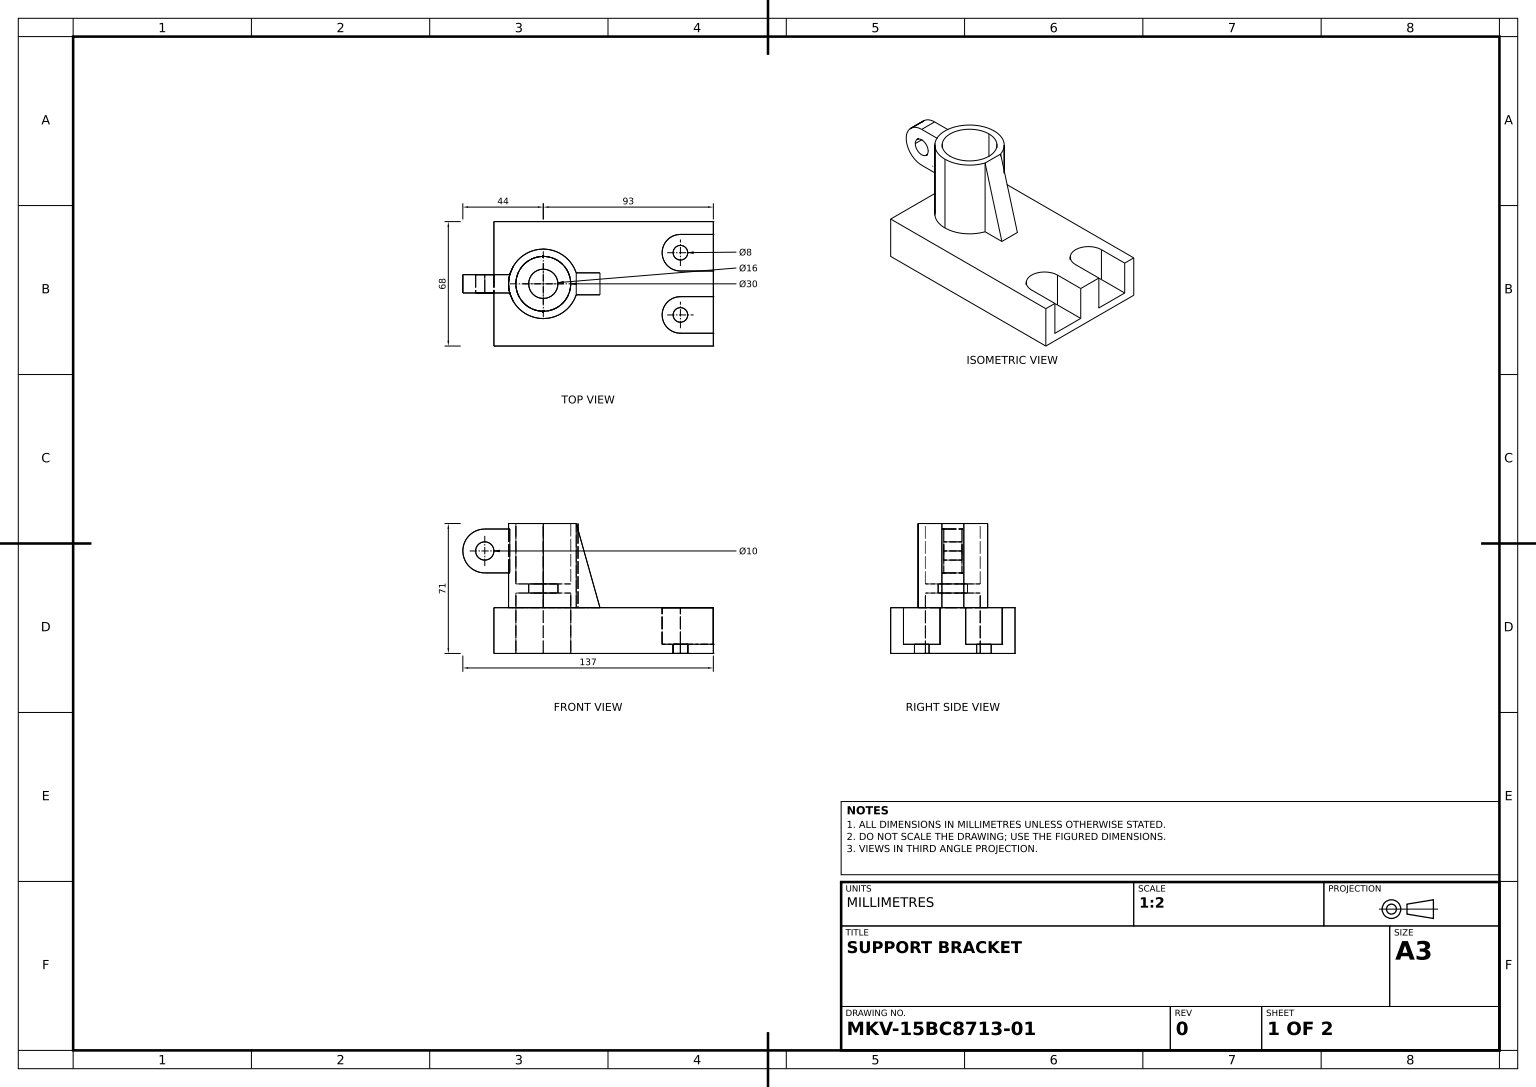
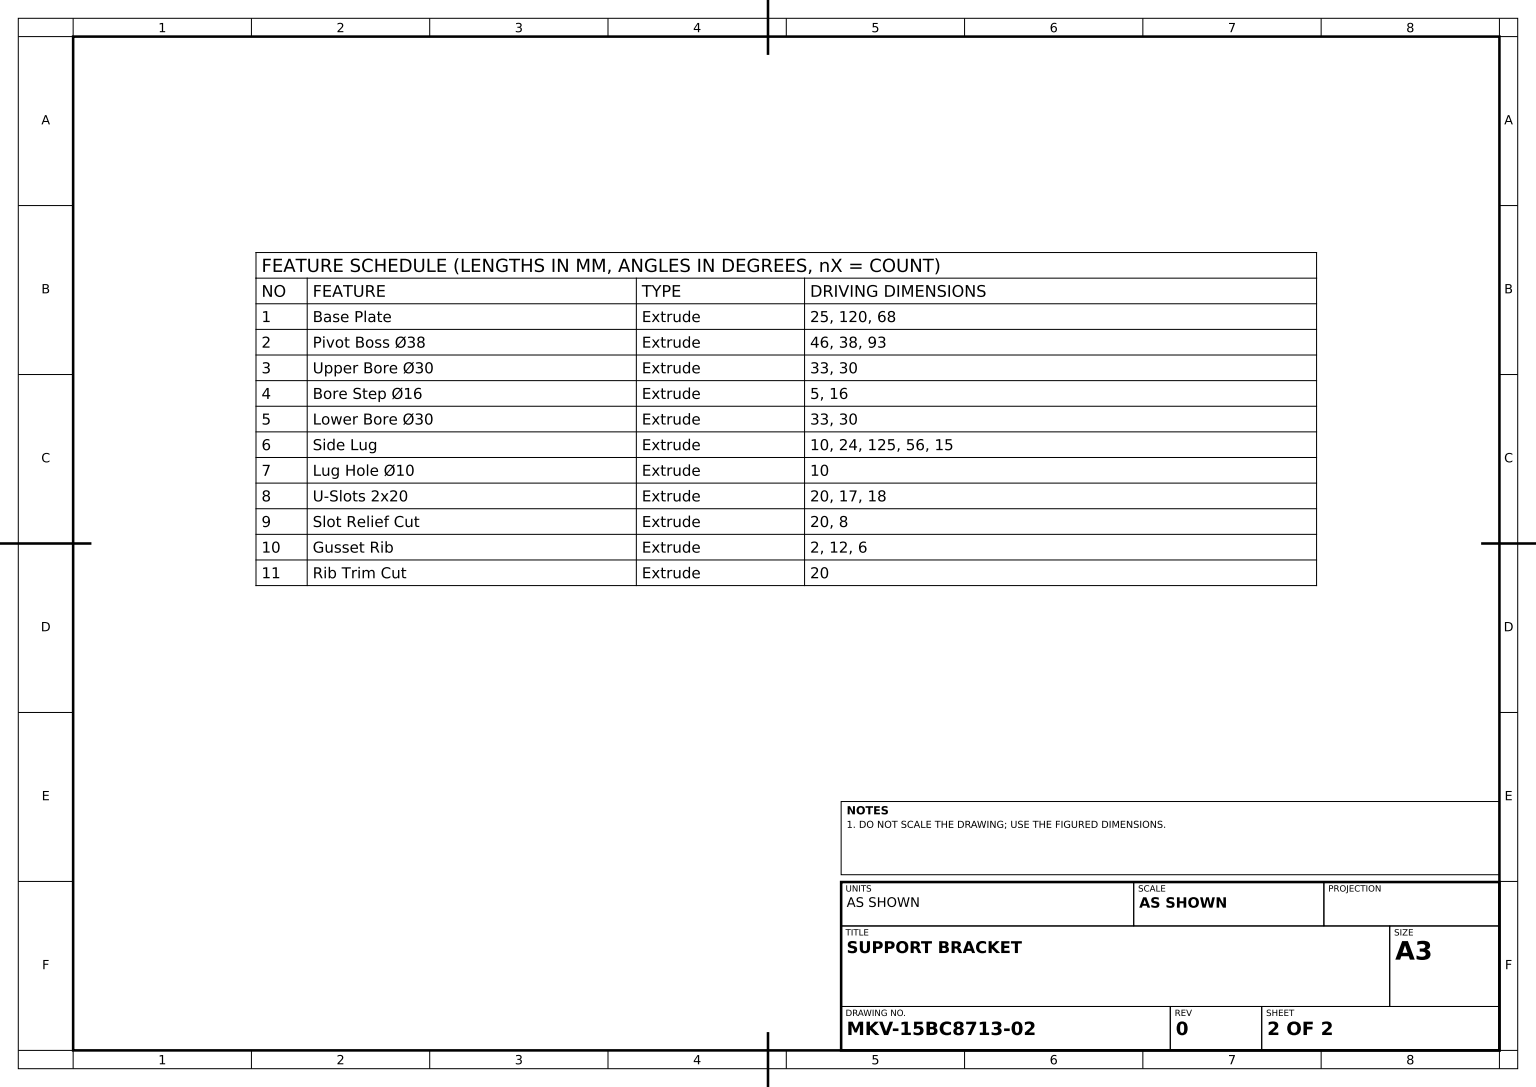
SolidWorks part; units mm, degrees
material "Plain Carbon Steel"
ref_plane "Front Plane" through (0, 0, 0) normal (0, 0, 1) x (1, 0, 0)
ref_plane "Top Plane" through (0, 0, 0) normal (0, 1, 0) x (1, 0, 0)
ref_plane "Right Plane" through (0, 0, 0) normal (1, 0, 0) x (0, 0, -1)
sketch "Base Plate Sketch" plane through (0, 0, 0) normal (0, 1, 0) x (1, 0, 0)
  line L1 (-60, -34) -> (60, -34)
  line L2 (-60, -34) -> (-60, 34)
  line L3 (-60, 34) -> (60, 34)
  line L4 (60, -34) -> (60, 34)
  line L5 (-60, -34) -> (60, 34) construction
  line L6 (-60, 34) -> (60, -34) construction
  point P0 (0, 0)
  dimension "D1" = 120
  dimension "D2" = 68
extrude "Base Plate" add sketch "Base Plate Sketch" along normal blind 25
sketch "Pivot Boss Sketch" plane through (0, 25, 0) normal (0, 1, 0) x (1, 0, 0)
  line L0 (60, -34) -> (60, 34) construction
  circle A0 centre (-33, 0) radius 19
  dimension "D1" = 38
  dimension "D2" = 93
extrude "Pivot Boss Ø38" add sketch "Pivot Boss Sketch" along normal blind 46
sketch "Upper Bore Sketch" plane through (0, 71, 0) normal (0, 1, 0) x (1, 0, 0)
  circle A0 centre (-33, 0) radius 15
  dimension "D1" = 30
extrude "Upper Bore Ø30" cut sketch "Upper Bore Sketch" against normal blind 33
sketch "Bore Step Sketch" plane through (0, 38, 0) normal (0, 1, 0) x (1, 0, 0)
  circle A0 centre (-33, 0) radius 8
  dimension "D1" = 16
extrude "Bore Step Ø16" cut sketch "Bore Step Sketch" against normal blind 5
sketch "Lower Bore Sketch" plane through (0, 33, 0) normal (0, 1, 0) x (1, 0, 0)
  circle A0 centre (-33, 0) radius 15
  dimension "D1" = 30
extrude "Lower Bore Ø30" cut sketch "Lower Bore Sketch" against normal blind 33
sketch "Side Lug Sketch" plane through (0, 0, 0) normal (0, 0, 1) x (1, 0, 0)
  line L0 (60, 25) -> (60, 0) construction
  line L1 (-60, 0) -> (60, 0) construction
  line L2 (-65, 68) -> (-50, 68)
  line L3 (-50, 68) -> (-50, 44)
  line L4 (-50, 44) -> (-65, 44)
  arc A0 (-65, 68) -> (-65, 44) centre (-65, 56) ccw
  dimension "D1" = 24
  dimension "D2" = 125
  dimension "D3" = 56
  dimension "D4" = 15
extrude "Side Lug" add sketch "Side Lug Sketch" along normal mid plane 10
sketch "Lug Hole Sketch" plane through (0, 0, 5) normal (0, 0, 1) x (1, 0, 0)
  circle A0 centre (-65, 56) radius 5
  dimension "D1" = 10
extrude "Lug Hole Ø10" cut sketch "Lug Hole Sketch" against normal blind 10
sketch "U-Slots Sketch" plane through (0, 25, 0) normal (0, 1, 0) x (1, 0, 0)
  line L0 (60, -34) -> (60, 34) construction
  line L1 (42, 27) -> (60, 27)
  line L2 (60, 27) -> (60, 7)
  line L3 (60, 7) -> (42, 7)
  line L4 (42, -7) -> (60, -7)
  line L5 (60, -7) -> (60, -27)
  line L6 (60, -27) -> (42, -27)
  arc A0 (42, 27) -> (42, 7) centre (42, 17) ccw
  arc A1 (42, -7) -> (42, -27) centre (42, -17) ccw
  dimension "D1" = 20
  dimension "D2" = 20
  dimension "D3" = 17
  dimension "D4" = 17
  dimension "D5" = 18
extrude "U-Slots 2x20" cut sketch "U-Slots Sketch" against normal blind 20
sketch "Slot Relief Sketch" plane through (0, 5, 0) normal (0, 1, 0) x (1, 0, 0)
  circle A0 centre (42, 17) radius 4
  circle A1 centre (42, -17) radius 4
  dimension "D1" = 8
extrude "Slot Relief Cut" cut sketch "Slot Relief Sketch" against normal blind 20
ref_plane "Rib Plane" through (-2, 0, 0) normal (1, 0, 0) x (0, 0, -1)
sketch "Gusset Rib Sketch" plane through (-2, 0, 0) normal (1, 0, 0) x (0, 0, -1)
  line L0 (15, 71) -> (-15, 71) construction
  line L1 (-6, 71) -> (6, 71)
  line L2 (-6, 71) -> (-6, 25)
  line L3 (-6, 25) -> (6, 25)
  line L4 (6, 71) -> (6, 25)
  line L5 (-7, 25) -> (7, 25) construction
  dimension "D1" = 12
  dimension "D2" = 6
extrude "Gusset Rib" add sketch "Gusset Rib Sketch" against normal up to next
sketch "Rib Trim Sketch" plane through (0, 0, 6) normal (0, 0, 1) x (1, 0, 0)
  line L0 (-14.9722, 71) -> (-2, 25)
  line L1 (-14.9722, 71) -> (-2, 71)
  line L2 (-2, 71) -> (-2, 25)
extrude "Rib Trim Cut" cut sketch "Rib Trim Sketch" against normal blind 20
